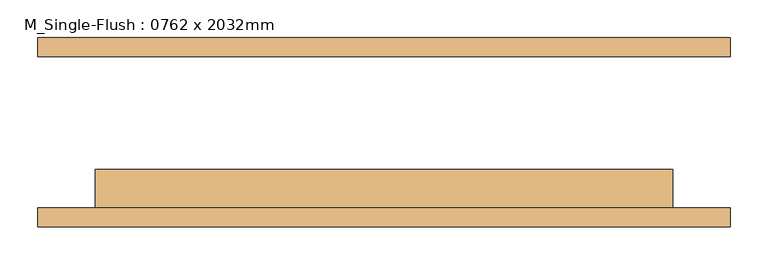
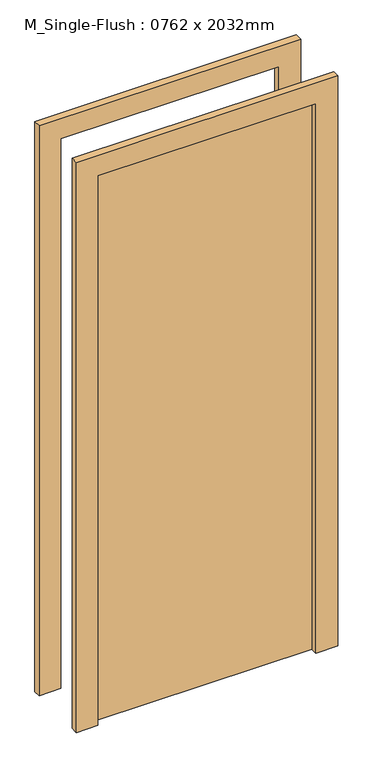
"""IFC4 building model written with IfcOpenShell, lengths in millimetres: door geometry, M_Single-Flush : 0762 x 2032mm."""

from ifc_helpers import new_model, si_unit, frame, origin, origin_with_axes, place, context, project, spatial, polyline, outline, extrude, source, transform, mapped, element, save


def m_single_flush_0762_x_2032mm_7341a4fb(model_context):
    return source(origin(), model_context, "Body", "SweptSolid", [
        extrude(outline(polyline([(2108.0, -457.0), (0.0, -457.0), (0.0, -381.0), (2032.0, -381.0), (2032.0, 381.0), (0.0, 381.0), (0.0, 457.0), (2108.0, 457.0), (2108.0, -457.0)])), frame((0.0, -125.0, 0.0), z_axis=(0.0, 1.0, 0.0), x_axis=(0.0, 0.0, 1.0)), (0.0, 0.0, 1.0), 25.0),
        extrude(outline(polyline([(2108.0, 457.0), (2108.0, -457.0), (0.0, -457.0), (0.0, -381.0), (2032.0, -381.0), (2032.0, 381.0), (0.0, 381.0), (0.0, 457.0), (2108.0, 457.0)])), frame((0.0, 100.0, 0.0), z_axis=(0.0, 1.0, 0.0), x_axis=(0.0, 0.0, 1.0)), (0.0, 0.0, 1.0), 25.0),
        extrude(outline(polyline([(381.0, -49.0), (381.0, -100.0), (-381.0, -100.0), (-381.0, -49.0), (381.0, -49.0)])), origin_with_axes(), (0.0, 0.0, 1.0), 2032.0),
    ])


if __name__ == "__main__":
    model = new_model("IFC4")
    model_context = context("Model", 3, world=origin())
    ifc_project = project(units=[si_unit("LENGTHUNIT", "METRE", prefix="MILLI")], contexts=[model_context])
    site = spatial("IfcSite", under=ifc_project)
    building = spatial("IfcBuilding", under=site)
    placement = place(None, origin())
    m_single_flush_0762_x_2032mm_shape = m_single_flush_0762_x_2032mm_7341a4fb(model_context)
    element("IfcDoor", 1, ObjectType="M_Single-Flush : 0762 x 2032mm", at=placement, inside=building, context=model_context, shape_type="MappedRepresentation", body=[
        mapped(m_single_flush_0762_x_2032mm_shape, transform((0.0, 0.0, 0.0), x_axis=(1.0, 0.0, 0.0), y_axis=(0.0, 1.0, 0.0), z_axis=(0.0, 0.0, 1.0))),
    ])
    save(model, "model.ifc")

# Revit data of these elements
# Type "M_Single-Flush : 0762 x 2032mm"
#   Type Mark = "19"
#   Thickness = 0' - 2.00787"
#   Height = 6' - 8"
#   Trim Projection Ext = 0' - 0.98425"
#   Trim Projection Int = 0' - 0.98425"
#   Trim Width = 0' - 2.99213"
#   Width = 2' - 6"
#   Door Material = Door - Panel
#   Frame Material = Door - Frame
#   Function = (empty or 0)
#   Wall Closure = (empty or 0)
# Element 1 (IfcDoor, "M_Single-Flush : 0762 x 2032mm")
#   Materials on its faces: "Door - Frame", "Door - Panel"
# Materials
#   "Door - Panel": class "Wood", colour RGB 114 82 51, transparency 0
#   "Door - Frame": colour RGB 153 76 43, transparency 0
